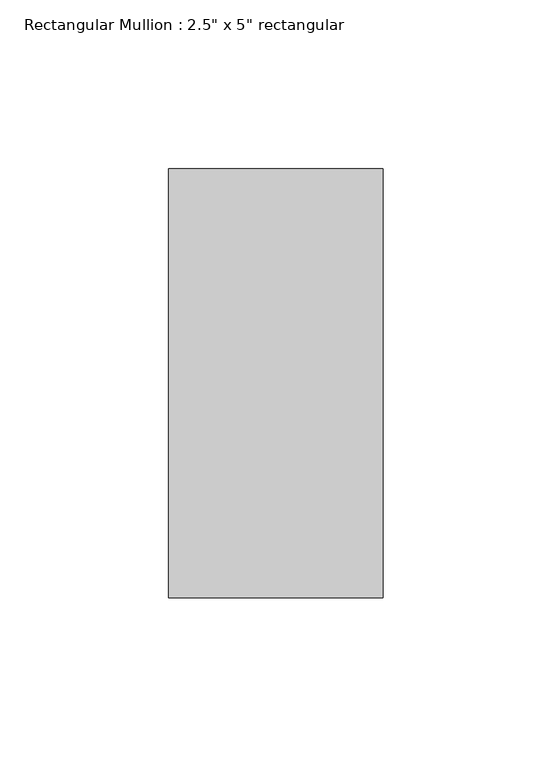
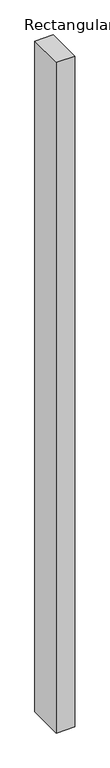
"""IFC4 building model written with IfcOpenShell, lengths in millimetres: member geometry."""

from ifc_helpers import new_model, si_unit, frame, origin, place, context, project, spatial, polyline, outline, extrude, source, transform, mapped, element, save


def member_f0fea5a5(model_context):
    return source(origin(), model_context, "Body", "SweptSolid", [
        extrude(outline(polyline([(31.75, 63.5), (31.75, -63.5), (-31.75, -63.5), (-31.75, 63.5), (31.75, 63.5)])), frame((0.0, 0.0, -2438.4), z_axis=(0.0, 0.0, 1.0), x_axis=(1.0, 0.0, 0.0)), (0.0, 0.0, 1.0), 2438.4),
    ])


if __name__ == "__main__":
    model = new_model("IFC4")
    model_context = context("Model", 3, world=origin())
    ifc_project = project(units=[si_unit("LENGTHUNIT", "METRE", prefix="MILLI")], contexts=[model_context])
    site = spatial("IfcSite", under=ifc_project)
    building = spatial("IfcBuilding", under=site)
    placement = place(None, origin())
    member_shape = member_f0fea5a5(model_context)
    element("IfcMember", 1, ObjectType="Rectangular Mullion : 2.5\" x 5\" rectangular", at=placement, inside=building, context=model_context, shape_type="MappedRepresentation", body=[
        mapped(member_shape, transform((0.0, 0.0, 0.0), x_axis=(1.0, 0.0, 0.0), y_axis=(0.0, 1.0, 0.0), z_axis=(0.0, 0.0, 1.0))),
    ])
    save(model, "model.ifc")

# Revit data of these elements
# Type "Rectangular Mullion : 2.5\" x 5\" rectangular"
#   built-in parameter 1007304 = 0.416667 (stored number, unit not read)
#   built-in parameter 1007301 = 0.104167 (stored number, unit not read)
#   built-in parameter 1007300 = 0.104167 (stored number, unit not read)
# Element 1 (IfcMember, "Rectangular Mullion : 2.5\" x 5\" rectangular")
#   Materials on its faces: "BLACK MATERIAL"
# Materials
#   "BLACK MATERIAL": class "Generic", colour RGB 120 120 120, transparency 0, Cost = 0
